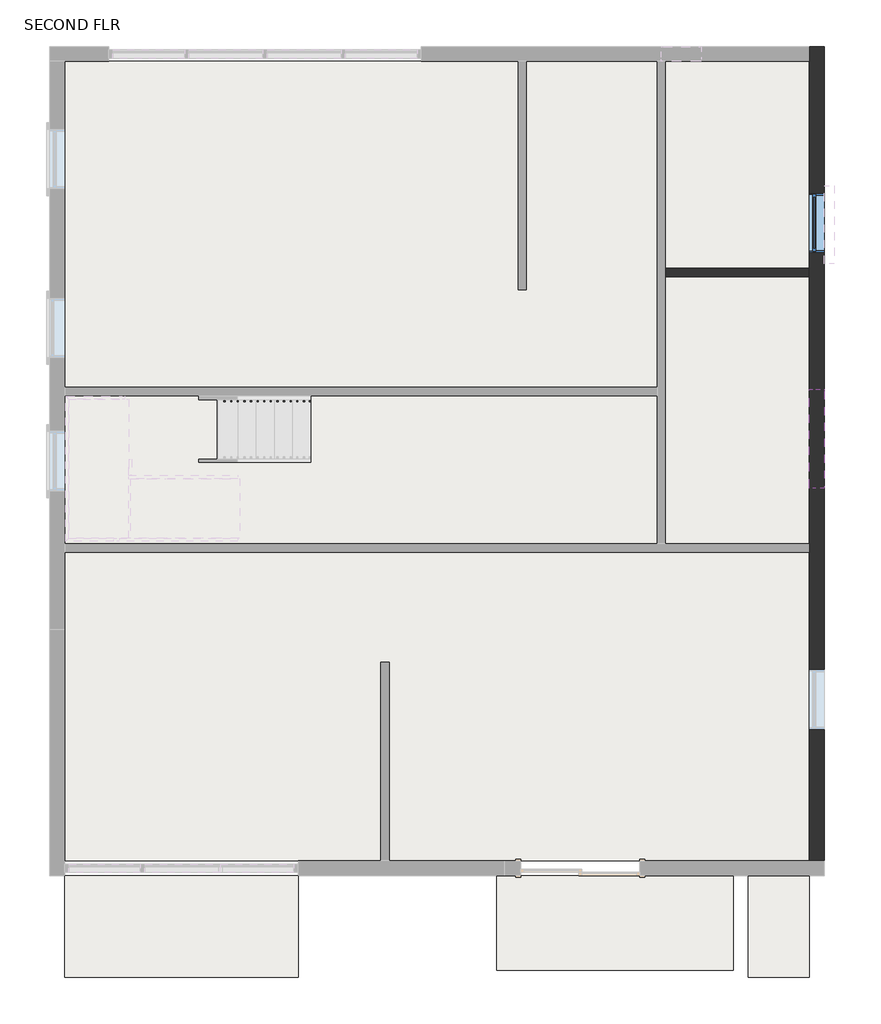
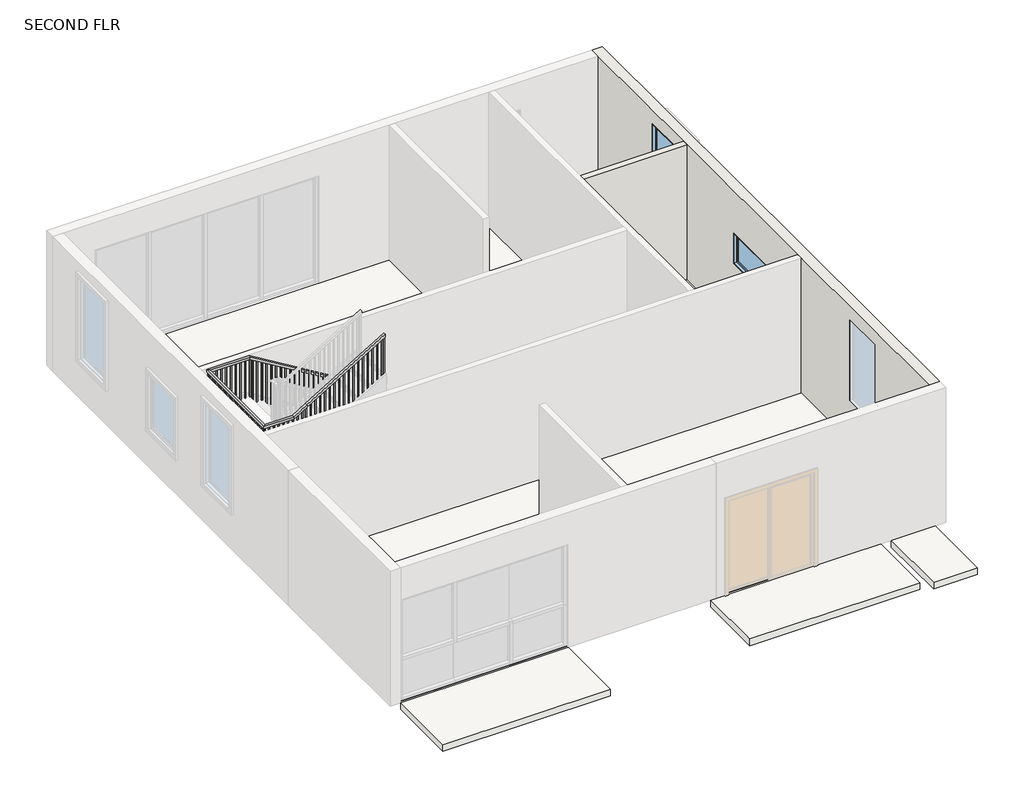
# One storey, part 2 of 3: 2 walls, 2 windows, 1 railing, 1 slab.
"""IFC4 building model written with IfcOpenShell, lengths in millimetres."""

from ifc_helpers import new_model, si_unit, frame, origin, place, context, project, spatial, polyline, outline, extrude, faceted_brep, transform, mapped, element, save
from components import window_2e8ca8a3, window_e88f44c6

model = new_model("IFC4")

# Units and contexts
model_context = context("Model", 3, world=origin())
ifc_project = project(units=[si_unit("LENGTHUNIT", "METRE", prefix="MILLI")], contexts=[model_context])

# Site, building, storey
site = spatial("IfcSite", under=ifc_project)
building = spatial("IfcBuilding", under=site)
storey = spatial("IfcBuildingStorey", under=building, Name="SECOND FLR", Elevation=6400.8)

# Railing
placement = place(None, origin())
element("IfcRailing", 1, ObjectType="Handrail - Rectangular", at=placement, inside=storey, context=model_context, shape_type="SolidModel", body=[
    faceted_brep([(-5990.8517085, 2868.2826226, 7789.3333333), (-5990.8517085, 2868.2826226, 7729.9318731), (-5990.8517085, 2919.0826226, 7729.9318731), (-5990.8517085, 2919.0826226, 7789.3333333), (-8784.8517085, 2868.2826226, 9482.6666667), (-8799.0441179, 2868.2826226, 9431.8666667), (-8799.0441179, 2919.0826226, 9431.8666667), (-8784.8517085, 2919.0826226, 9482.6666667), (-9648.4517085, 2868.2826226, 9482.6666667), (-9648.4517085, 2868.2826226, 9431.8666667), (-9699.2517085, 2919.0826226, 9431.8666667), (-9699.2517085, 2919.0826226, 9482.6666667), (-9648.4517085, 842.8165128, 9482.6666667), (-9648.4517085, 842.8165128, 9431.8666667), (-9699.2517085, 792.0165128, 9431.8666667), (-9699.2517085, 792.0165128, 9482.6666667), (-9064.2517085, 842.8165128, 9482.6666667), (-9050.0592991, 842.8165128, 9431.8666667), (-9050.0592991, 792.0165128, 9431.8666667), (-9064.2517085, 792.0165128, 9482.6666667), (-8784.8517085, 842.8165128, 9652.0), (-8758.5219813, 842.8165128, 9608.5559502), (-8758.5219813, 792.0165128, 9608.5559502), (-8784.8517085, 792.0165128, 9652.0), (-7108.4517085, 842.8165128, 10668.0), (-7108.4517085, 792.0165128, 10668.0), (-7108.4517085, 792.0165128, 10608.5985397), (-7108.4517085, 842.8165128, 10608.5985397)], [[[0, 1, 2, 3]], [[1, 0, 4, 5]], [[2, 1, 5, 6]], [[3, 2, 6, 7]], [[0, 3, 7, 4]], [[5, 4, 8, 9]], [[6, 5, 9, 10]], [[7, 6, 10, 11]], [[4, 7, 11, 8]], [[9, 8, 12, 13]], [[10, 9, 13, 14]], [[11, 10, 14, 15]], [[8, 11, 15, 12]], [[13, 12, 16, 17]], [[14, 13, 17, 18]], [[15, 14, 18, 19]], [[12, 15, 19, 16]], [[17, 16, 20, 21]], [[18, 17, 21, 22]], [[19, 18, 22, 23]], [[16, 19, 23, 20]], [[24, 25, 26, 27]], [[21, 20, 24, 27]], [[22, 21, 27, 26]], [[23, 22, 26, 25]], [[20, 23, 25, 24]]]),
    extrude(outline(polyline([(10583.5833882, -7149.7267085), (10572.0379337, -7168.7767085), (9584.2666667, -7168.7767085), (9584.2666667, -7149.7267085), (10583.5833882, -7149.7267085)])), frame((0.0, 807.8915128, 0.0), z_axis=(0.0, 1.0, 0.0), x_axis=(0.0, 0.0, 1.0)), (0.0, 0.0, 1.0), 19.05),
    extrude(outline(polyline([(10522.0076307, -7251.3267085), (10510.4621761, -7270.3767085), (9584.2666667, -7270.3767085), (9584.2666667, -7251.3267085), (10522.0076307, -7251.3267085)])), frame((0.0, 807.8915128, 0.0), z_axis=(0.0, 1.0, 0.0), x_axis=(0.0, 0.0, 1.0)), (0.0, 0.0, 1.0), 19.05),
    extrude(outline(polyline([(10460.4318731, -7352.9267085), (10448.8864185, -7371.9767085), (9584.2666667, -7371.9767085), (9584.2666667, -7352.9267085), (10460.4318731, -7352.9267085)])), frame((0.0, 807.8915128, 0.0), z_axis=(0.0, 1.0, 0.0), x_axis=(0.0, 0.0, 1.0)), (0.0, 0.0, 1.0), 19.05),
    extrude(outline(polyline([(10398.8561155, -7454.5267085), (10387.310661, -7473.5767085), (9414.9333333, -7473.5767085), (9414.9333333, -7454.5267085), (10398.8561155, -7454.5267085)])), frame((0.0, 807.8915128, 0.0), z_axis=(0.0, 1.0, 0.0), x_axis=(0.0, 0.0, 1.0)), (0.0, 0.0, 1.0), 19.05),
    extrude(outline(polyline([(10337.2803579, -7556.1267085), (10325.7349034, -7575.1767085), (9414.9333333, -7575.1767085), (9414.9333333, -7556.1267085), (10337.2803579, -7556.1267085)])), frame((0.0, 807.8915128, 0.0), z_axis=(0.0, 1.0, 0.0), x_axis=(0.0, 0.0, 1.0)), (0.0, 0.0, 1.0), 19.05),
    extrude(outline(polyline([(10275.7046004, -7657.7267085), (10264.1591458, -7676.7767085), (9414.9333333, -7676.7767085), (9414.9333333, -7657.7267085), (10275.7046004, -7657.7267085)])), frame((0.0, 807.8915128, 0.0), z_axis=(0.0, 1.0, 0.0), x_axis=(0.0, 0.0, 1.0)), (0.0, 0.0, 1.0), 19.05),
    extrude(outline(polyline([(10214.1288428, -7759.3267085), (10202.5833882, -7778.3767085), (9245.6, -7778.3767085), (9245.6, -7759.3267085), (10214.1288428, -7759.3267085)])), frame((0.0, 807.8915128, 0.0), z_axis=(0.0, 1.0, 0.0), x_axis=(0.0, 0.0, 1.0)), (0.0, 0.0, 1.0), 19.05),
    extrude(outline(polyline([(10152.5530852, -7860.9267085), (10141.0076307, -7879.9767085), (9245.6, -7879.9767085), (9245.6, -7860.9267085), (10152.5530852, -7860.9267085)])), frame((0.0, 807.8915128, 0.0), z_axis=(0.0, 1.0, 0.0), x_axis=(0.0, 0.0, 1.0)), (0.0, 0.0, 1.0), 19.05),
    extrude(outline(polyline([(10090.9773276, -7962.5267085), (10079.4318731, -7981.5767085), (9076.2666667, -7981.5767085), (9076.2666667, -7962.5267085), (10090.9773276, -7962.5267085)])), frame((0.0, 807.8915128, 0.0), z_axis=(0.0, 1.0, 0.0), x_axis=(0.0, 0.0, 1.0)), (0.0, 0.0, 1.0), 19.05),
    extrude(outline(polyline([(10029.4015701, -8064.1267085), (10017.8561155, -8083.1767085), (9076.2666667, -8083.1767085), (9076.2666667, -8064.1267085), (10029.4015701, -8064.1267085)])), frame((0.0, 807.8915128, 0.0), z_axis=(0.0, 1.0, 0.0), x_axis=(0.0, 0.0, 1.0)), (0.0, 0.0, 1.0), 19.05),
    extrude(outline(polyline([(9967.8258125, -8165.7267085), (9956.2803579, -8184.7767085), (9076.2666667, -8184.7767085), (9076.2666667, -8165.7267085), (9967.8258125, -8165.7267085)])), frame((0.0, 807.8915128, 0.0), z_axis=(0.0, 1.0, 0.0), x_axis=(0.0, 0.0, 1.0)), (0.0, 0.0, 1.0), 19.05),
    extrude(outline(polyline([(9906.2500549, -8267.3267085), (9894.7046004, -8286.3767085), (8906.9333333, -8286.3767085), (8906.9333333, -8267.3267085), (9906.2500549, -8267.3267085)])), frame((0.0, 807.8915128, 0.0), z_axis=(0.0, 1.0, 0.0), x_axis=(0.0, 0.0, 1.0)), (0.0, 0.0, 1.0), 19.05),
    extrude(outline(polyline([(9844.6742973, -8368.9267085), (9833.1288428, -8387.9767085), (8906.9333333, -8387.9767085), (8906.9333333, -8368.9267085), (9844.6742973, -8368.9267085)])), frame((0.0, 807.8915128, 0.0), z_axis=(0.0, 1.0, 0.0), x_axis=(0.0, 0.0, 1.0)), (0.0, 0.0, 1.0), 19.05),
    extrude(outline(polyline([(9783.0985397, -8470.5267085), (9771.5530852, -8489.5767085), (8906.9333333, -8489.5767085), (8906.9333333, -8470.5267085), (9783.0985397, -8470.5267085)])), frame((0.0, 807.8915128, 0.0), z_axis=(0.0, 1.0, 0.0), x_axis=(0.0, 0.0, 1.0)), (0.0, 0.0, 1.0), 19.05),
    extrude(outline(polyline([(9721.5227822, -8572.1267085), (9709.9773276, -8591.1767085), (8737.6, -8591.1767085), (8737.6, -8572.1267085), (9721.5227822, -8572.1267085)])), frame((0.0, 807.8915128, 0.0), z_axis=(0.0, 1.0, 0.0), x_axis=(0.0, 0.0, 1.0)), (0.0, 0.0, 1.0), 19.05),
    extrude(outline(polyline([(9659.9470246, -8673.7267085), (9648.40157, -8692.7767085), (8737.6, -8692.7767085), (8737.6, -8673.7267085), (9659.9470246, -8673.7267085)])), frame((0.0, 807.8915128, 0.0), z_axis=(0.0, 1.0, 0.0), x_axis=(0.0, 0.0, 1.0)), (0.0, 0.0, 1.0), 19.05),
    extrude(outline(polyline([(9552.1894488, -8851.5267085), (9540.6439943, -8870.5767085), (8568.2666667, -8870.5767085), (8568.2666667, -8851.5267085), (9552.1894488, -8851.5267085)])), frame((0.0, 807.8915128, 0.0), z_axis=(0.0, 1.0, 0.0), x_axis=(0.0, 0.0, 1.0)), (0.0, 0.0, 1.0), 19.05),
    extrude(outline(polyline([(9490.6136913, -8953.1267085), (9479.0682367, -8972.1767085), (8568.2666667, -8972.1767085), (8568.2666667, -8953.1267085), (9490.6136913, -8953.1267085)])), frame((0.0, 807.8915128, 0.0), z_axis=(0.0, 1.0, 0.0), x_axis=(0.0, 0.0, 1.0)), (0.0, 0.0, 1.0), 19.05),
    extrude(outline(polyline([(-9073.7767085, 807.8915128), (-9073.7767085, 826.9415128), (-9054.7267085, 826.9415128), (-9054.7267085, 807.8915128), (-9073.7767085, 807.8915128)])), frame((0.0, 0.0, 8568.2666667), z_axis=(0.0, 0.0, 1.0), x_axis=(1.0, 0.0, 0.0)), (0.0, 0.0, 1.0), 863.6),
    extrude(outline(polyline([(-9175.3767085, 807.8915128), (-9175.3767085, 826.9415128), (-9156.3267085, 826.9415128), (-9156.3267085, 807.8915128), (-9175.3767085, 807.8915128)])), frame((0.0, 0.0, 8568.2666667), z_axis=(0.0, 0.0, 1.0), x_axis=(1.0, 0.0, 0.0)), (0.0, 0.0, 1.0), 863.6),
    extrude(outline(polyline([(-9276.9767085, 807.8915128), (-9276.9767085, 826.9415128), (-9257.9267085, 826.9415128), (-9257.9267085, 807.8915128), (-9276.9767085, 807.8915128)])), frame((0.0, 0.0, 8568.2666667), z_axis=(0.0, 0.0, 1.0), x_axis=(1.0, 0.0, 0.0)), (0.0, 0.0, 1.0), 863.6),
    extrude(outline(polyline([(-9378.5767085, 807.8915128), (-9378.5767085, 826.9415128), (-9359.5267085, 826.9415128), (-9359.5267085, 807.8915128), (-9378.5767085, 807.8915128)])), frame((0.0, 0.0, 8568.2666667), z_axis=(0.0, 0.0, 1.0), x_axis=(1.0, 0.0, 0.0)), (0.0, 0.0, 1.0), 863.6),
    extrude(outline(polyline([(-9480.1767085, 807.8915128), (-9480.1767085, 826.9415128), (-9461.1267085, 826.9415128), (-9461.1267085, 807.8915128), (-9480.1767085, 807.8915128)])), frame((0.0, 0.0, 8568.2666667), z_axis=(0.0, 0.0, 1.0), x_axis=(1.0, 0.0, 0.0)), (0.0, 0.0, 1.0), 863.6),
    extrude(outline(polyline([(-9581.7767085, 807.8915128), (-9581.7767085, 826.9415128), (-9562.7267085, 826.9415128), (-9562.7267085, 807.8915128), (-9581.7767085, 807.8915128)])), frame((0.0, 0.0, 8568.2666667), z_axis=(0.0, 0.0, 1.0), x_axis=(1.0, 0.0, 0.0)), (0.0, 0.0, 1.0), 863.6),
    extrude(outline(polyline([(-9683.3767085, 871.2076226), (-9664.3267085, 871.2076226), (-9664.3267085, 852.1576226), (-9683.3767085, 852.1576226), (-9683.3767085, 871.2076226)])), frame((0.0, 0.0, 8568.2666667), z_axis=(0.0, 0.0, 1.0), x_axis=(1.0, 0.0, 0.0)), (0.0, 0.0, 1.0), 863.6),
    extrude(outline(polyline([(-9683.3767085, 972.8076226), (-9664.3267085, 972.8076226), (-9664.3267085, 953.7576226), (-9683.3767085, 953.7576226), (-9683.3767085, 972.8076226)])), frame((0.0, 0.0, 8568.2666667), z_axis=(0.0, 0.0, 1.0), x_axis=(1.0, 0.0, 0.0)), (0.0, 0.0, 1.0), 863.6),
    extrude(outline(polyline([(-9683.3767085, 1074.4076226), (-9664.3267085, 1074.4076226), (-9664.3267085, 1055.3576226), (-9683.3767085, 1055.3576226), (-9683.3767085, 1074.4076226)])), frame((0.0, 0.0, 8568.2666667), z_axis=(0.0, 0.0, 1.0), x_axis=(1.0, 0.0, 0.0)), (0.0, 0.0, 1.0), 863.6),
    extrude(outline(polyline([(-9683.3767085, 1176.0076226), (-9664.3267085, 1176.0076226), (-9664.3267085, 1156.9576226), (-9683.3767085, 1156.9576226), (-9683.3767085, 1176.0076226)])), frame((0.0, 0.0, 8568.2666667), z_axis=(0.0, 0.0, 1.0), x_axis=(1.0, 0.0, 0.0)), (0.0, 0.0, 1.0), 863.6),
    extrude(outline(polyline([(-9683.3767085, 1277.6076226), (-9664.3267085, 1277.6076226), (-9664.3267085, 1258.5576226), (-9683.3767085, 1258.5576226), (-9683.3767085, 1277.6076226)])), frame((0.0, 0.0, 8568.2666667), z_axis=(0.0, 0.0, 1.0), x_axis=(1.0, 0.0, 0.0)), (0.0, 0.0, 1.0), 863.6),
    extrude(outline(polyline([(-9683.3767085, 1379.2076226), (-9664.3267085, 1379.2076226), (-9664.3267085, 1360.1576226), (-9683.3767085, 1360.1576226), (-9683.3767085, 1379.2076226)])), frame((0.0, 0.0, 8568.2666667), z_axis=(0.0, 0.0, 1.0), x_axis=(1.0, 0.0, 0.0)), (0.0, 0.0, 1.0), 863.6),
    extrude(outline(polyline([(-9683.3767085, 1480.8076226), (-9664.3267085, 1480.8076226), (-9664.3267085, 1461.7576226), (-9683.3767085, 1461.7576226), (-9683.3767085, 1480.8076226)])), frame((0.0, 0.0, 8568.2666667), z_axis=(0.0, 0.0, 1.0), x_axis=(1.0, 0.0, 0.0)), (0.0, 0.0, 1.0), 863.6),
    extrude(outline(polyline([(-9683.3767085, 1582.4076226), (-9664.3267085, 1582.4076226), (-9664.3267085, 1563.3576226), (-9683.3767085, 1563.3576226), (-9683.3767085, 1582.4076226)])), frame((0.0, 0.0, 8568.2666667), z_axis=(0.0, 0.0, 1.0), x_axis=(1.0, 0.0, 0.0)), (0.0, 0.0, 1.0), 863.6),
    extrude(outline(polyline([(-9683.3767085, 1684.0076226), (-9664.3267085, 1684.0076226), (-9664.3267085, 1664.9576226), (-9683.3767085, 1664.9576226), (-9683.3767085, 1684.0076226)])), frame((0.0, 0.0, 8568.2666667), z_axis=(0.0, 0.0, 1.0), x_axis=(1.0, 0.0, 0.0)), (0.0, 0.0, 1.0), 863.6),
    extrude(outline(polyline([(-9683.3767085, 1785.6076226), (-9664.3267085, 1785.6076226), (-9664.3267085, 1766.5576226), (-9683.3767085, 1766.5576226), (-9683.3767085, 1785.6076226)])), frame((0.0, 0.0, 8568.2666667), z_axis=(0.0, 0.0, 1.0), x_axis=(1.0, 0.0, 0.0)), (0.0, 0.0, 1.0), 863.6),
    extrude(outline(polyline([(-9683.3767085, 1887.2076226), (-9664.3267085, 1887.2076226), (-9664.3267085, 1868.1576226), (-9683.3767085, 1868.1576226), (-9683.3767085, 1887.2076226)])), frame((0.0, 0.0, 8568.2666667), z_axis=(0.0, 0.0, 1.0), x_axis=(1.0, 0.0, 0.0)), (0.0, 0.0, 1.0), 863.6),
    extrude(outline(polyline([(-9683.3767085, 1988.8076226), (-9664.3267085, 1988.8076226), (-9664.3267085, 1969.7576226), (-9683.3767085, 1969.7576226), (-9683.3767085, 1988.8076226)])), frame((0.0, 0.0, 8568.2666667), z_axis=(0.0, 0.0, 1.0), x_axis=(1.0, 0.0, 0.0)), (0.0, 0.0, 1.0), 863.6),
    extrude(outline(polyline([(-9683.3767085, 2090.4076226), (-9664.3267085, 2090.4076226), (-9664.3267085, 2071.3576226), (-9683.3767085, 2071.3576226), (-9683.3767085, 2090.4076226)])), frame((0.0, 0.0, 8568.2666667), z_axis=(0.0, 0.0, 1.0), x_axis=(1.0, 0.0, 0.0)), (0.0, 0.0, 1.0), 863.6),
    extrude(outline(polyline([(-9683.3767085, 2192.0076226), (-9664.3267085, 2192.0076226), (-9664.3267085, 2172.9576226), (-9683.3767085, 2172.9576226), (-9683.3767085, 2192.0076226)])), frame((0.0, 0.0, 8568.2666667), z_axis=(0.0, 0.0, 1.0), x_axis=(1.0, 0.0, 0.0)), (0.0, 0.0, 1.0), 863.6),
    extrude(outline(polyline([(-9683.3767085, 2293.6076226), (-9664.3267085, 2293.6076226), (-9664.3267085, 2274.5576226), (-9683.3767085, 2274.5576226), (-9683.3767085, 2293.6076226)])), frame((0.0, 0.0, 8568.2666667), z_axis=(0.0, 0.0, 1.0), x_axis=(1.0, 0.0, 0.0)), (0.0, 0.0, 1.0), 863.6),
    extrude(outline(polyline([(-9683.3767085, 2395.2076226), (-9664.3267085, 2395.2076226), (-9664.3267085, 2376.1576226), (-9683.3767085, 2376.1576226), (-9683.3767085, 2395.2076226)])), frame((0.0, 0.0, 8568.2666667), z_axis=(0.0, 0.0, 1.0), x_axis=(1.0, 0.0, 0.0)), (0.0, 0.0, 1.0), 863.6),
    extrude(outline(polyline([(-9683.3767085, 2496.8076226), (-9664.3267085, 2496.8076226), (-9664.3267085, 2477.7576226), (-9683.3767085, 2477.7576226), (-9683.3767085, 2496.8076226)])), frame((0.0, 0.0, 8568.2666667), z_axis=(0.0, 0.0, 1.0), x_axis=(1.0, 0.0, 0.0)), (0.0, 0.0, 1.0), 863.6),
    extrude(outline(polyline([(-9683.3767085, 2598.4076226), (-9664.3267085, 2598.4076226), (-9664.3267085, 2579.3576226), (-9683.3767085, 2579.3576226), (-9683.3767085, 2598.4076226)])), frame((0.0, 0.0, 8568.2666667), z_axis=(0.0, 0.0, 1.0), x_axis=(1.0, 0.0, 0.0)), (0.0, 0.0, 1.0), 863.6),
    extrude(outline(polyline([(-9683.3767085, 2700.0076226), (-9664.3267085, 2700.0076226), (-9664.3267085, 2680.9576226), (-9683.3767085, 2680.9576226), (-9683.3767085, 2700.0076226)])), frame((0.0, 0.0, 8568.2666667), z_axis=(0.0, 0.0, 1.0), x_axis=(1.0, 0.0, 0.0)), (0.0, 0.0, 1.0), 863.6),
    extrude(outline(polyline([(-9683.3767085, 2801.6076226), (-9664.3267085, 2801.6076226), (-9664.3267085, 2782.5576226), (-9683.3767085, 2782.5576226), (-9683.3767085, 2801.6076226)])), frame((0.0, 0.0, 8568.2666667), z_axis=(0.0, 0.0, 1.0), x_axis=(1.0, 0.0, 0.0)), (0.0, 0.0, 1.0), 863.6),
    extrude(outline(polyline([(-9588.1267085, 2903.2076226), (-9588.1267085, 2884.1576226), (-9607.1767085, 2884.1576226), (-9607.1767085, 2903.2076226), (-9588.1267085, 2903.2076226)])), frame((0.0, 0.0, 8568.2666667), z_axis=(0.0, 0.0, 1.0), x_axis=(1.0, 0.0, 0.0)), (0.0, 0.0, 1.0), 863.6),
    extrude(outline(polyline([(-9486.5267085, 2903.2076226), (-9486.5267085, 2884.1576226), (-9505.5767085, 2884.1576226), (-9505.5767085, 2903.2076226), (-9486.5267085, 2903.2076226)])), frame((0.0, 0.0, 8568.2666667), z_axis=(0.0, 0.0, 1.0), x_axis=(1.0, 0.0, 0.0)), (0.0, 0.0, 1.0), 863.6),
    extrude(outline(polyline([(-9384.9267085, 2903.2076226), (-9384.9267085, 2884.1576226), (-9403.9767085, 2884.1576226), (-9403.9767085, 2903.2076226), (-9384.9267085, 2903.2076226)])), frame((0.0, 0.0, 8568.2666667), z_axis=(0.0, 0.0, 1.0), x_axis=(1.0, 0.0, 0.0)), (0.0, 0.0, 1.0), 863.6),
    extrude(outline(polyline([(-9283.3267085, 2903.2076226), (-9283.3267085, 2884.1576226), (-9302.3767085, 2884.1576226), (-9302.3767085, 2903.2076226), (-9283.3267085, 2903.2076226)])), frame((0.0, 0.0, 8568.2666667), z_axis=(0.0, 0.0, 1.0), x_axis=(1.0, 0.0, 0.0)), (0.0, 0.0, 1.0), 863.6),
    extrude(outline(polyline([(-9181.7267085, 2903.2076226), (-9181.7267085, 2884.1576226), (-9200.7767085, 2884.1576226), (-9200.7767085, 2903.2076226), (-9181.7267085, 2903.2076226)])), frame((0.0, 0.0, 8568.2666667), z_axis=(0.0, 0.0, 1.0), x_axis=(1.0, 0.0, 0.0)), (0.0, 0.0, 1.0), 863.6),
    extrude(outline(polyline([(-9080.1267085, 2903.2076226), (-9080.1267085, 2884.1576226), (-9099.1767085, 2884.1576226), (-9099.1767085, 2903.2076226), (-9080.1267085, 2903.2076226)])), frame((0.0, 0.0, 8568.2666667), z_axis=(0.0, 0.0, 1.0), x_axis=(1.0, 0.0, 0.0)), (0.0, 0.0, 1.0), 863.6),
    extrude(outline(polyline([(-8978.5267085, 2903.2076226), (-8978.5267085, 2884.1576226), (-8997.5767085, 2884.1576226), (-8997.5767085, 2903.2076226), (-8978.5267085, 2903.2076226)])), frame((0.0, 0.0, 8568.2666667), z_axis=(0.0, 0.0, 1.0), x_axis=(1.0, 0.0, 0.0)), (0.0, 0.0, 1.0), 863.6),
    extrude(outline(polyline([(-8876.9267085, 2903.2076226), (-8876.9267085, 2884.1576226), (-8895.9767085, 2884.1576226), (-8895.9767085, 2903.2076226), (-8876.9267085, 2903.2076226)])), frame((0.0, 0.0, 8568.2666667), z_axis=(0.0, 0.0, 1.0), x_axis=(1.0, 0.0, 0.0)), (0.0, 0.0, 1.0), 863.6),
    extrude(outline(polyline([(9386.7046004, -8724.5267085), (9398.2500549, -8743.5767085), (8398.9333333, -8743.5767085), (8398.9333333, -8724.5267085), (9386.7046004, -8724.5267085)])), frame((0.0, 2884.1576226, 0.0), z_axis=(0.0, 1.0, 0.0), x_axis=(0.0, 0.0, 1.0)), (0.0, 0.0, 1.0), 19.05),
    extrude(outline(polyline([(9325.1288428, -8622.9267085), (9336.6742973, -8641.9767085), (8398.9333333, -8641.9767085), (8398.9333333, -8622.9267085), (9325.1288428, -8622.9267085)])), frame((0.0, 2884.1576226, 0.0), z_axis=(0.0, 1.0, 0.0), x_axis=(0.0, 0.0, 1.0)), (0.0, 0.0, 1.0), 19.05),
    extrude(outline(polyline([(9263.5530852, -8521.3267085), (9275.0985397, -8540.3767085), (8398.9333333, -8540.3767085), (8398.9333333, -8521.3267085), (9263.5530852, -8521.3267085)])), frame((0.0, 2884.1576226, 0.0), z_axis=(0.0, 1.0, 0.0), x_axis=(0.0, 0.0, 1.0)), (0.0, 0.0, 1.0), 19.05),
    extrude(outline(polyline([(9201.9773276, -8419.7267085), (9213.5227822, -8438.7767085), (8229.6, -8438.7767085), (8229.6, -8419.7267085), (9201.9773276, -8419.7267085)])), frame((0.0, 2884.1576226, 0.0), z_axis=(0.0, 1.0, 0.0), x_axis=(0.0, 0.0, 1.0)), (0.0, 0.0, 1.0), 19.05),
    extrude(outline(polyline([(9140.40157, -8318.1267085), (9151.9470246, -8337.1767085), (8229.6, -8337.1767085), (8229.6, -8318.1267085), (9140.40157, -8318.1267085)])), frame((0.0, 2884.1576226, 0.0), z_axis=(0.0, 1.0, 0.0), x_axis=(0.0, 0.0, 1.0)), (0.0, 0.0, 1.0), 19.05),
    extrude(outline(polyline([(9078.8258125, -8216.5267085), (9090.371267, -8235.5767085), (8229.6, -8235.5767085), (8229.6, -8216.5267085), (9078.8258125, -8216.5267085)])), frame((0.0, 2884.1576226, 0.0), z_axis=(0.0, 1.0, 0.0), x_axis=(0.0, 0.0, 1.0)), (0.0, 0.0, 1.0), 19.05),
    extrude(outline(polyline([(9017.2500549, -8114.9267085), (9028.7955094, -8133.9767085), (8060.2666667, -8133.9767085), (8060.2666667, -8114.9267085), (9017.2500549, -8114.9267085)])), frame((0.0, 2884.1576226, 0.0), z_axis=(0.0, 1.0, 0.0), x_axis=(0.0, 0.0, 1.0)), (0.0, 0.0, 1.0), 19.05),
    extrude(outline(polyline([(8955.6742973, -8013.3267085), (8967.2197519, -8032.3767085), (8060.2666667, -8032.3767085), (8060.2666667, -8013.3267085), (8955.6742973, -8013.3267085)])), frame((0.0, 2884.1576226, 0.0), z_axis=(0.0, 1.0, 0.0), x_axis=(0.0, 0.0, 1.0)), (0.0, 0.0, 1.0), 19.05),
    extrude(outline(polyline([(8894.0985397, -7911.7267085), (8905.6439943, -7930.7767085), (7890.9333333, -7930.7767085), (7890.9333333, -7911.7267085), (8894.0985397, -7911.7267085)])), frame((0.0, 2884.1576226, 0.0), z_axis=(0.0, 1.0, 0.0), x_axis=(0.0, 0.0, 1.0)), (0.0, 0.0, 1.0), 19.05),
    extrude(outline(polyline([(8832.5227822, -7810.1267085), (8844.0682367, -7829.1767085), (7890.9333333, -7829.1767085), (7890.9333333, -7810.1267085), (8832.5227822, -7810.1267085)])), frame((0.0, 2884.1576226, 0.0), z_axis=(0.0, 1.0, 0.0), x_axis=(0.0, 0.0, 1.0)), (0.0, 0.0, 1.0), 19.05),
    extrude(outline(polyline([(8770.9470246, -7708.5267085), (8782.4924791, -7727.5767085), (7890.9333333, -7727.5767085), (7890.9333333, -7708.5267085), (8770.9470246, -7708.5267085)])), frame((0.0, 2884.1576226, 0.0), z_axis=(0.0, 1.0, 0.0), x_axis=(0.0, 0.0, 1.0)), (0.0, 0.0, 1.0), 19.05),
    extrude(outline(polyline([(8709.371267, -7606.9267085), (8720.9167216, -7625.9767085), (7721.6, -7625.9767085), (7721.6, -7606.9267085), (8709.371267, -7606.9267085)])), frame((0.0, 2884.1576226, 0.0), z_axis=(0.0, 1.0, 0.0), x_axis=(0.0, 0.0, 1.0)), (0.0, 0.0, 1.0), 19.05),
    extrude(outline(polyline([(8647.7955094, -7505.3267085), (8659.340964, -7524.3767085), (7721.6, -7524.3767085), (7721.6, -7505.3267085), (8647.7955094, -7505.3267085)])), frame((0.0, 2884.1576226, 0.0), z_axis=(0.0, 1.0, 0.0), x_axis=(0.0, 0.0, 1.0)), (0.0, 0.0, 1.0), 19.05),
    extrude(outline(polyline([(8586.2197519, -7403.7267085), (8597.7652064, -7422.7767085), (7721.6, -7422.7767085), (7721.6, -7403.7267085), (8586.2197519, -7403.7267085)])), frame((0.0, 2884.1576226, 0.0), z_axis=(0.0, 1.0, 0.0), x_axis=(0.0, 0.0, 1.0)), (0.0, 0.0, 1.0), 19.05),
    extrude(outline(polyline([(8524.6439943, -7302.1267085), (8536.1894488, -7321.1767085), (7552.2666667, -7321.1767085), (7552.2666667, -7302.1267085), (8524.6439943, -7302.1267085)])), frame((0.0, 2884.1576226, 0.0), z_axis=(0.0, 1.0, 0.0), x_axis=(0.0, 0.0, 1.0)), (0.0, 0.0, 1.0), 19.05),
    extrude(outline(polyline([(8463.0682367, -7200.5267085), (8474.6136913, -7219.5767085), (7552.2666667, -7219.5767085), (7552.2666667, -7200.5267085), (8463.0682367, -7200.5267085)])), frame((0.0, 2884.1576226, 0.0), z_axis=(0.0, 1.0, 0.0), x_axis=(0.0, 0.0, 1.0)), (0.0, 0.0, 1.0), 19.05),
    extrude(outline(polyline([(8401.4924791, -7098.9267085), (8413.0379337, -7117.9767085), (7552.2666667, -7117.9767085), (7552.2666667, -7098.9267085), (8401.4924791, -7098.9267085)])), frame((0.0, 2884.1576226, 0.0), z_axis=(0.0, 1.0, 0.0), x_axis=(0.0, 0.0, 1.0)), (0.0, 0.0, 1.0), 19.05),
    extrude(outline(polyline([(8339.9167216, -6997.3267085), (8351.4621761, -7016.3767085), (7382.9333333, -7016.3767085), (7382.9333333, -6997.3267085), (8339.9167216, -6997.3267085)])), frame((0.0, 2884.1576226, 0.0), z_axis=(0.0, 1.0, 0.0), x_axis=(0.0, 0.0, 1.0)), (0.0, 0.0, 1.0), 19.05),
    extrude(outline(polyline([(8278.340964, -6895.7267085), (8289.8864185, -6914.7767085), (7382.9333333, -6914.7767085), (7382.9333333, -6895.7267085), (8278.340964, -6895.7267085)])), frame((0.0, 2884.1576226, 0.0), z_axis=(0.0, 1.0, 0.0), x_axis=(0.0, 0.0, 1.0)), (0.0, 0.0, 1.0), 19.05),
    extrude(outline(polyline([(8216.7652064, -6794.1267085), (8228.310661, -6813.1767085), (7213.6, -6813.1767085), (7213.6, -6794.1267085), (8216.7652064, -6794.1267085)])), frame((0.0, 2884.1576226, 0.0), z_axis=(0.0, 1.0, 0.0), x_axis=(0.0, 0.0, 1.0)), (0.0, 0.0, 1.0), 19.05),
    extrude(outline(polyline([(8155.1894488, -6692.5267085), (8166.7349034, -6711.5767085), (7213.6, -6711.5767085), (7213.6, -6692.5267085), (8155.1894488, -6692.5267085)])), frame((0.0, 2884.1576226, 0.0), z_axis=(0.0, 1.0, 0.0), x_axis=(0.0, 0.0, 1.0)), (0.0, 0.0, 1.0), 19.05),
    extrude(outline(polyline([(8093.6136913, -6590.9267085), (8105.1591458, -6609.9767085), (7213.6, -6609.9767085), (7213.6, -6590.9267085), (8093.6136913, -6590.9267085)])), frame((0.0, 2884.1576226, 0.0), z_axis=(0.0, 1.0, 0.0), x_axis=(0.0, 0.0, 1.0)), (0.0, 0.0, 1.0), 19.05),
    extrude(outline(polyline([(8032.0379337, -6489.3267085), (8043.5833882, -6508.3767085), (7044.2666667, -6508.3767085), (7044.2666667, -6489.3267085), (8032.0379337, -6489.3267085)])), frame((0.0, 2884.1576226, 0.0), z_axis=(0.0, 1.0, 0.0), x_axis=(0.0, 0.0, 1.0)), (0.0, 0.0, 1.0), 19.05),
    extrude(outline(polyline([(7970.4621761, -6387.7267085), (7982.0076307, -6406.7767085), (7044.2666667, -6406.7767085), (7044.2666667, -6387.7267085), (7970.4621761, -6387.7267085)])), frame((0.0, 2884.1576226, 0.0), z_axis=(0.0, 1.0, 0.0), x_axis=(0.0, 0.0, 1.0)), (0.0, 0.0, 1.0), 19.05),
    extrude(outline(polyline([(7908.8864185, -6286.1267085), (7920.4318731, -6305.1767085), (7044.2666667, -6305.1767085), (7044.2666667, -6286.1267085), (7908.8864185, -6286.1267085)])), frame((0.0, 2884.1576226, 0.0), z_axis=(0.0, 1.0, 0.0), x_axis=(0.0, 0.0, 1.0)), (0.0, 0.0, 1.0), 19.05),
    extrude(outline(polyline([(7847.310661, -6184.5267085), (7858.8561155, -6203.5767085), (6874.9333333, -6203.5767085), (6874.9333333, -6184.5267085), (7847.310661, -6184.5267085)])), frame((0.0, 2884.1576226, 0.0), z_axis=(0.0, 1.0, 0.0), x_axis=(0.0, 0.0, 1.0)), (0.0, 0.0, 1.0), 19.05),
    extrude(outline(polyline([(7785.7349034, -6082.9267085), (7797.2803579, -6101.9767085), (6874.9333333, -6101.9767085), (6874.9333333, -6082.9267085), (7785.7349034, -6082.9267085)])), frame((0.0, 2884.1576226, 0.0), z_axis=(0.0, 1.0, 0.0), x_axis=(0.0, 0.0, 1.0)), (0.0, 0.0, 1.0), 19.05),
    extrude(outline(polyline([(9598.371267, -8775.3267085), (9586.8258125, -8794.3767085), (8568.2666667, -8794.3767085), (8568.2666667, -8775.3267085), (9598.371267, -8775.3267085)])), frame((0.0, 807.8915128, 0.0), z_axis=(0.0, 1.0, 0.0), x_axis=(0.0, 0.0, 1.0)), (0.0, 0.0, 1.0), 19.05),
    extrude(outline(polyline([(-9683.3767085, 826.9415128), (-9664.3267085, 826.9415128), (-9664.3267085, 807.8915128), (-9683.3767085, 807.8915128), (-9683.3767085, 826.9415128)])), frame((0.0, 0.0, 8568.2666667), z_axis=(0.0, 0.0, 1.0), x_axis=(1.0, 0.0, 0.0)), (0.0, 0.0, 1.0), 863.6),
    extrude(outline(polyline([(-9664.3267085, 2903.2076226), (-9664.3267085, 2884.1576226), (-9683.3767085, 2884.1576226), (-9683.3767085, 2903.2076226), (-9664.3267085, 2903.2076226)])), frame((0.0, 0.0, 8568.2666667), z_axis=(0.0, 0.0, 1.0), x_axis=(1.0, 0.0, 0.0)), (0.0, 0.0, 1.0), 863.6),
    extrude(outline(polyline([(9417.4924791, -8775.3267085), (9429.0379337, -8794.3767085), (8568.2666667, -8794.3767085), (8568.2666667, -8775.3267085), (9417.4924791, -8775.3267085)])), frame((0.0, 2884.1576226, 0.0), z_axis=(0.0, 1.0, 0.0), x_axis=(0.0, 0.0, 1.0)), (0.0, 0.0, 1.0), 19.05),
    extrude(outline(polyline([(10608.5985397, -7108.4517085), (10597.0530852, -7127.5017085), (9584.2666667, -7127.5017085), (9584.2666667, -7108.4517085), (10608.5985397, -7108.4517085)])), frame((0.0, 807.8915128, 0.0), z_axis=(0.0, 1.0, 0.0), x_axis=(0.0, 0.0, 1.0)), (0.0, 0.0, 1.0), 19.05),
    extrude(outline(polyline([(7729.9318731, -5990.8517085), (7741.4773276, -6009.9017085), (6874.9333333, -6009.9017085), (6874.9333333, -5990.8517085), (7729.9318731, -5990.8517085)])), frame((0.0, 2884.1576226, 0.0), z_axis=(0.0, 1.0, 0.0), x_axis=(0.0, 0.0, 1.0)), (0.0, 0.0, 1.0), 19.05),
])

# Slab
element("IfcSlab", 2, ObjectType="MARBLE FLOORING 6\"", at=placement, inside=storey, context=model_context, shape_type="SweptSolid", body=[
    extrude(outline(polyline([(-670.7781265, 2976.7857468), (-670.7781265, 703.1165128), (-9763.9781265, 703.1165128), (-9763.9781265, 2976.7857468), (-670.7781265, 2976.7857468)])), frame((0.0, 0.0, 6248.4), z_axis=(0.0, 0.0, 1.0), x_axis=(1.0, 0.0, 0.0)), (0.0, 0.0, 1.0), 152.4),
    extrude(outline(polyline([(1666.0218735, 4805.5857468), (1666.0218735, 703.1165128), (-543.7781265, 703.1165128), (-543.7781265, 4805.5857468), (1666.0218735, 4805.5857468)])), frame((0.0, 0.0, 6248.4), z_axis=(0.0, 0.0, 1.0), x_axis=(1.0, 0.0, 0.0)), (0.0, 0.0, 1.0), 152.4),
    extrude(outline(polyline([(1666.0218735, 8107.5857468), (1666.0218735, 4932.5857468), (-543.7781265, 4932.5857468), (-543.7781265, 8107.5857468), (1666.0218735, 8107.5857468)])), frame((0.0, 0.0, 6248.4), z_axis=(0.0, 0.0, 1.0), x_axis=(1.0, 0.0, 0.0)), (0.0, 0.0, 1.0), 152.4),
    extrude(outline(polyline([(497.6218735, -4389.2142532), (497.6218735, -5837.0142532), (-3134.5781265, -5837.0142532), (-3134.5781265, -4389.2142532), (497.6218735, -4389.2142532)])), frame((0.0, 0.0, 6248.4), z_axis=(0.0, 0.0, 1.0), x_axis=(1.0, 0.0, 0.0)), (0.0, 0.0, 1.0), 152.4),
    extrude(outline(polyline([(-4912.5781265, -4160.6142532), (-9763.9781265, -4160.6142532), (-9763.9781265, 576.1165128), (1666.0218735, 576.1165128), (1666.0218735, -4160.6142532), (-4785.5781265, -4160.6142532), (-4785.5781265, -1112.6142532), (-4912.5781265, -1112.6142532), (-4912.5781265, -4160.6142532)])), frame((0.0, 0.0, 6248.4), z_axis=(0.0, 0.0, 1.0), x_axis=(1.0, 0.0, 0.0)), (0.0, 0.0, 1.0), 152.4),
    extrude(outline(polyline([(-9763.9781265, 8107.5857468), (-2804.3781265, 8107.5857468), (-2804.3781265, 4602.3857468), (-2677.3781265, 4602.3857468), (-2677.3781265, 8107.5857468), (-670.7781265, 8107.5857468), (-670.7781265, 3103.7857468), (-9763.9781265, 3103.7857468), (-9763.9781265, 8107.5857468)])), frame((0.0, 0.0, 6248.4), z_axis=(0.0, 0.0, 1.0), x_axis=(1.0, 0.0, 0.0)), (0.0, 0.0, 1.0), 152.4),
    extrude(outline(polyline([(-9763.9781265, -4389.2142532), (-6182.5781265, -4389.2142532), (-6182.5781265, -5951.3142532), (-9763.9781265, -5951.3142532), (-9763.9781265, -4389.2142532)])), frame((0.0, 0.0, 6248.4), z_axis=(0.0, 0.0, 1.0), x_axis=(1.0, 0.0, 0.0)), (0.0, 0.0, 1.0), 152.4),
    extrude(outline(polyline([(1666.0218735, -4389.2142532), (1666.0218735, -5951.3142532), (726.2218735, -5951.3142532), (726.2218735, -4389.2142532), (1666.0218735, -4389.2142532)])), frame((0.0, 0.0, 6248.4), z_axis=(0.0, 0.0, 1.0), x_axis=(1.0, 0.0, 0.0)), (0.0, 0.0, 1.0), 152.4),
])

# Walls
element("IfcWall", 3, ObjectType="INNER WALL THICKNESS 5\"", at=placement, inside=storey, context=model_context, shape_type="SweptSolid", body=[
    extrude(outline(polyline([(1666.0218735, 4805.5857468), (-543.7781265, 4805.5857468), (-543.7781265, 4932.5857468), (1666.0218735, 4932.5857468), (1666.0218735, 4805.5857468)])), frame((0.0, 0.0, 6400.8), z_axis=(0.0, 0.0, 1.0), x_axis=(1.0, 0.0, 0.0)), (0.0, 0.0, 1.0), 3048.0),
])
element("IfcWall", 4, ObjectType="OUTER WALL THICKNESS 9\"", at=placement, inside=storey, context=model_context, shape_type="Brep", body=[
    faceted_brep([(1894.6218735, -4160.6142532, 6400.8), (1894.6218735, 8336.1857468, 6400.8), (1894.6218735, 8336.1857468, 9448.8), (1894.6218735, -4160.6142532, 9448.8), (1894.6218735, 6088.2857468, 9144.0), (1894.6218735, 6088.2857468, 7315.2), (1894.6218735, 5173.8857468, 7315.2), (1894.6218735, 5173.8857468, 9144.0), (1894.6218735, -1226.9142532, 9144.0), (1894.6218735, -1226.9142532, 7315.2), (1894.6218735, -2141.3142532, 7315.2), (1894.6218735, -2141.3142532, 9144.0), (1894.6218735, 3078.0165128, 8496.2767967), (1894.6218735, 3078.0165128, 7810.4767967), (1894.6218735, 1554.0165128, 7810.4767967), (1894.6218735, 1554.0165128, 8496.2767967), (1666.0218735, -4160.6142532, 6400.8), (1666.0218735, -4160.6142532, 9448.8), (1666.0218735, 576.1165128, 9448.8), (1666.0218735, 703.1165128, 9448.8), (1666.0218735, 4805.5857468, 9448.8), (1666.0218735, 4932.5857468, 9448.8), (1666.0218735, 8107.5857468, 9448.8), (1666.0218735, 8336.1857468, 9448.8), (1666.0218735, 8336.1857468, 6400.8), (1666.0218735, 8107.5857468, 6400.8), (1666.0218735, 4932.5857468, 6400.8), (1666.0218735, 4805.5857468, 6400.8), (1666.0218735, 703.1165128, 6400.8), (1666.0218735, 576.1165128, 6400.8), (1666.0218735, 6088.2857468, 9144.0), (1666.0218735, 5173.8857468, 9144.0), (1666.0218735, 5173.8857468, 7315.2), (1666.0218735, 6088.2857468, 7315.2), (1666.0218735, -1226.9142532, 9144.0), (1666.0218735, -2141.3142532, 9144.0), (1666.0218735, -2141.3142532, 7315.2), (1666.0218735, -1226.9142532, 7315.2), (1666.0218735, 3078.0165128, 8496.2767967), (1666.0218735, 1554.0165128, 8496.2767967), (1666.0218735, 1554.0165128, 7810.4767967), (1666.0218735, 3078.0165128, 7810.4767967)], [[[0, 1, 2, 3], [4, 5, 6, 7], [8, 9, 10, 11], [12, 13, 14, 15]], [[16, 17, 18, 19, 20, 21, 22, 23, 24, 25, 26, 27, 28, 29], [30, 31, 32, 33], [34, 35, 36, 37], [38, 39, 40, 41]], [[1, 0, 16, 29, 28, 27, 26, 25, 24]], [[3, 2, 23, 22, 21, 20, 19, 18, 17]], [[0, 3, 17, 16]], [[2, 1, 24, 23]], [[5, 4, 30, 33]], [[6, 5, 33, 32]], [[7, 6, 32, 31]], [[4, 7, 31, 30]], [[9, 8, 34, 37]], [[10, 9, 37, 36]], [[11, 10, 36, 35]], [[8, 11, 35, 34]], [[13, 12, 38, 41]], [[14, 13, 41, 40]], [[15, 14, 40, 39]], [[12, 15, 39, 38]]]),
])

# Windows
window_shape = window_2e8ca8a3(model_context)
element("IfcWindow", 5, ObjectType="Fixed : window 3' x 6\"", at=placement, inside=storey, context=model_context, shape_type="MappedRepresentation", body=[
    mapped(window_shape, transform((1780.3218735, 5669.1857468, 6400.8), x_axis=(0.0, 1.0, 0.0), y_axis=(-1.0, 0.0, 0.0), z_axis=(0.0, 0.0, 1.0))),
])
window_2_shape = window_e88f44c6(model_context)
element("IfcWindow", 6, ObjectType="Fixed : window length 5' x 2'3\"", at=placement, inside=storey, context=model_context, shape_type="MappedRepresentation", body=[
    mapped(window_2_shape, transform((1780.3218735, 2354.1165128, 6896.0767967), x_axis=(0.0, 1.0, 0.0), y_axis=(-1.0, 0.0, 0.0), z_axis=(0.0, 0.0, 1.0))),
])

save(model, "model.ifc")

# Revit data of these elements
# Type "Handrail - Rectangular"
#   Assembly Code = "C2010400"
#   built-in parameter 1008612 = 0.0416667 (stored number, unit not read)
#   built-in parameter 1008611 = 0.0416667 (stored number, unit not read)
#   built-in parameter 1008609 = 0.333333 (stored number, unit not read)
#   built-in parameter 1008604 = 0.166667 (stored number, unit not read)
#   built-in parameter 1008603 = 0.166667 (stored number, unit not read)
#   Railing Height = 3' - 0"
#   built-in parameter 1008630 = 2
#   built-in parameter 1008610 = 2
#   built-in parameter 1008618 = Baluster - Square : 3/4"
# Type "MARBLE FLOORING 6\""
#   Assembly Code = "B1010"
#   Function = 0
#   Layers, outside or top first: 0' - 6" "MARBLE FLOORING" (function 1)
# Type "INNER WALL THICKNESS 5\""
#   Assembly Code = "B2010"
#   Layers, outside or top first: 0' - 5" "WALL PAINT" (function 1)
# Type "OUTER WALL THICKNESS 9\""
#   Assembly Code = "B2010"
#   Layers, outside or top first: 0' - 9" "WALL PAINT" (function 1)
# Type "Fixed : window 3' x 6\""
#   Type Mark = "26"
#   Construction Type Id = "GSP4R"
#   Assembly Code = "B2020100"
#   Analytic Construction = "1/8 in Pilkington single glazing"
#   Visual Light Transmittance = 0.9
#   Solar Heat Gain Coefficient = 0.78
#   Heat Transfer Coefficient (U) = 0.6496 BTU/(h·ft²·°F)
#   Height = 6' - 0"
#   Default Sill Height = 3' - 0"
#   Width = 3' - 0"
#   Window Inset = 0' - 2"
#   Define Thermal Properties by = 1
#   Glass Pane Material = Glass
#   Sash Material = Sash
#   Wall Closure = (empty or 0)
# Type "Fixed : window length 5' x 2'3\""
#   Type Mark = "28"
#   Construction Type Id = "GSP4R"
#   Assembly Code = "B2020100"
#   Analytic Construction = "1/8 in Pilkington single glazing"
#   Visual Light Transmittance = 0.9
#   Solar Heat Gain Coefficient = 0.78
#   Heat Transfer Coefficient (U) = 0.6496 BTU/(h·ft²·°F)
#   Height = 2' - 3"
#   Default Sill Height = 3' - 0"
#   Width = 5' - 0"
#   Window Inset = 0' - 2"
#   Define Thermal Properties by = 1
#   Glass Pane Material = Glass
#   Sash Material = Sash
#   Wall Closure = (empty or 0)
# Element 1 (IfcRailing, "Handrail - Rectangular")
#   Phase Created = New Construction
# Element 2 (IfcSlab, "MARBLE FLOORING 6\"")
#   Height Offset From Level = 0' - 0"
#   Phase Created = New Construction
#   Materials on its faces: "MARBLE FLOORING"
# Element 3 (IfcWall, "INNER WALL THICKNESS 5\"")
#   Top Offset = 0' - 0"
#   Base Offset = 0' - 0"
#   Unconnected Height = 10' - 0"
#   wall height = 10' - 0"
#   Phase Created = New Construction
#   Base Constraint = SECOND FLR
#   Materials on its faces: "WALL PAINT"
# Element 4 (IfcWall, "OUTER WALL THICKNESS 9\"")
#   Top Offset = 0' - 0"
#   Base Offset = 0' - 0"
#   Unconnected Height = 10' - 0"
#   wall height = 10' - 0"
#   Phase Created = New Construction
#   Base Constraint = SECOND FLR
#   Materials on its faces: "WALL PAINT"
# Element 5 (IfcWindow, "Fixed : window 3' x 6\"")
#   Mark = "12"
#   Phase Created = New Construction
#   Materials on its faces: "Sash", "Glass"
# Element 6 (IfcWindow, "Fixed : window length 5' x 2'3\"")
#   Mark = "16"
#   Phase Created = New Construction
#   Materials on its faces: "Sash", "Glass"
# Materials
#   "MARBLE FLOORING": class "Generic", colour RGB 120 120 120, transparency 0, Cost = 0
#   "WALL PAINT": class "Generic", colour RGB 120 120 120, transparency 0, Cost = 0
#   "Glass": class "Glass", colour RGB 0 128 192, transparency 0.75, Description = "Soda Lime Glass", Cost = 0
#   "Sash": class "Wood", colour RGB 224 178 126, transparency 0, Cost = 0
